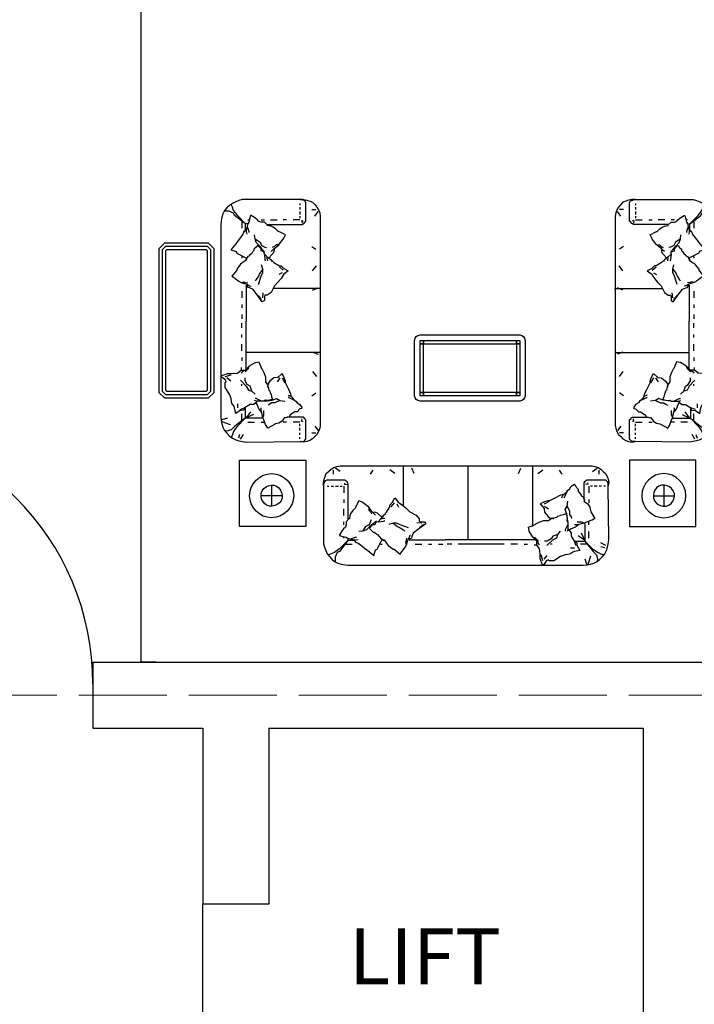
# Model space of a CAD drawing. Units: inches. Extents: x -113 to 5399, y -1393 to 3302.
# Tile 37 of 40: x 3412 to 3504, y 2903 to 3038. Entities that reach past the tile are written whole.
import ezdxf

# ---------------------------------------------------------------- set-up
doc = ezdxf.new("R2010")
doc.units = ezdxf.units.IN
doc.header["$MEASUREMENT"] = 0
doc.linetypes.add('ACAD_ISO02W100', pattern=[15, 12, -3])
doc.layers.add('24', color=7, linetype='Continuous')
for name, color, linetype, lineweight in [('A-ANNO-DIMS', 254, 'Continuous', 18), ('A-AREA-IDEN', 4, 'Continuous', 18), ('doors', 2, 'Continuous', 25), ('furniture', 131, 'Continuous', 18), ('GRIDS', 7, 'ACAD_ISO02W100', 13), ('walls', 1, 'Continuous', 25)]:
    doc.layers.add(name, color=color, linetype=linetype, lineweight=lineweight)
doc.styles.get("Standard").update_dxf_attribs({"font": 'arial.ttf'})
doc.dimstyles.get("Standard").update_dxf_attribs({"dimtxt": 6, "dimasz": 0.18, "dimexe": 0.18, "dimexo": 0.0625, "dimgap": 0.09, "dimtad": 0, "dimtih": 1, "dimtoh": 1, "dimdec": 1, "dimzin": 0, "dimdsep": 46, "dimlunit": 4, "dimtxsty": 'Standard', "dimblk": 'ARCHTICK', "dimcen": 0.09, "dimadec": 0, "dimazin": 0, "dimtfac": 1, "dimtdec": 1, "dimtofl": 0, "dimtmove": 0, "dimatfit": 3, "dimfxl": 1, "dimtolj": 1, "dimtzin": 0, "dimarcsym": 0})

# ---------------------------------------------------------------- blocks, each defined once
blk = doc.blocks.new('*U3')
for p, q in [((0, 0), (0, -6)), ((36, 0), (36, -6))]:
    blk.add_line(p, q)
blk.add_lwpolyline([(0, 0), (0, 36), (1.75, 36), (1.75, 0)], close=True)
blk.add_arc((0, 0), 36, 0, 90)
blk = doc.blocks.new('DL13712')
at = {"layer": '24'}
for p, q in [((33, 28.5), (-34, 28.5)), ((33.5, -29.5), (-10, -29.5))]:
    blk.add_line(p, q, dxfattribs=at)
blk = doc.blocks.new('DL13976')
at = {"layer": '24'}
for p, q in [((-10.5, 16.5), (-7, 18.5)), ((-7, 18.5), (-3.5, 19.5)), ((-3.5, 19.5), (0.5, 20)), ((0.5, 20), (4.5, 19.5)), ((4.5, 19.5), (8, 18.5)), ((8, 18.5), (11.5, 16.5)), ((-18, 7.5), (-16, 11)), ((-16, 11), (-13.5, 14)), ((-13.5, 14), (-10.5, 16.5)), ((-4.5, 8), (-2.5, 9)), ((-2.5, 9), (0, 9.5)), ((0, 9.5), (2.5, 9.5)), ((0.5, -9.5), (0.5, 9.5)), ((2.5, 9.5), (5, 8.5)), ((11.5, 16.5), (14.5, 14)), ((14.5, 14), (17, 11)), ((17, 11), (19, 7.5)), ((-19.5, 0), (-19, 4)), ((-19, -4), (-19.5, 0)), ((-19, 4), (-18, 7.5)), ((-9, 2), (-8, 4.5)), ((-9, -0.5), (-9, 2)), ((-9, 0), (10, 0)), ((-8, 4.5), (-6.5, 6.5)), ((-6.5, 6.5), (-4.5, 8)), ((-5.5, 0), (6.5, 0)), ((0.5, -6), (0.5, 6)), ((5, 8.5), (7, 7)), ((7, 7), (8.5, 5)), ((8.5, 5), (9.5, 3)), ((9.5, 3), (10, 0.5)), ((10, 0.5), (10, -2)), ((19, 7.5), (20, 4)), ((20, 4), (20.5, 0)), ((20.5, 0), (20, -4)), ((-18, -7.5), (-19, -4)), ((-16, -11), (-18, -7.5)), ((-8.5, -3), (-9, -0.5)), ((-7.5, -5), (-8.5, -3)), ((-6, -7), (-7.5, -5)), ((-4, -8.5), (-6, -7)), ((-1.5, -9.5), (-4, -8.5)), ((5.5, -8), (3.5, -9)), ((7.5, -6.5), (5.5, -8)), ((9, -4.5), (7.5, -6.5)), ((10, -2), (9, -4.5)), ((19, -7.5), (17, -11)), ((20, -4), (19, -7.5)), ((-13.5, -14), (-16, -11)), ((-10.5, -16.5), (-13.5, -14)), ((-7, -18.5), (-10.5, -16.5)), ((1, -9.5), (-1.5, -9.5)), ((3.5, -9), (1, -9.5)), ((11.5, -16.5), (8, -18.5)), ((14.5, -14), (11.5, -16.5)), ((17, -11), (14.5, -14)), ((-3.5, -19.5), (-7, -18.5)), ((0.5, -20), (-3.5, -19.5)), ((4.5, -19.5), (0.5, -20)), ((8, -18.5), (4.5, -19.5))]:
    blk.add_line(p, q, dxfattribs=at)
blk = doc.blocks.new('DL13329')
at = {"layer": '24'}
for p, q in [((0, 0), (0, -60)), ((60, 0), (0, 0)), ((60, -60), (60, 0)), ((0, -60), (60, -60))]:
    blk.add_line(p, q, dxfattribs=at)
blk = doc.blocks.new('DL13303')
at = {"layer": '24'}
for p, q in [((-70, 20), (-65, 25)), ((-70, -20), (-70, 20)), ((-67, 19), (-64, 22)), ((-67, -19), (-67, 19)), ((-65, 25), (65, 25)), ((-64, 22), (64, 22)), ((-64, 18), (-63, 19)), ((-64, -18), (-64, 18)), ((-63, 19), (63, 19)), ((63, 19), (64, 18)), ((64, 22), (67, 19)), ((64, 18), (64, -18)), ((65, 25), (70, 20)), ((67, 19), (67, -19)), ((70, 20), (70, -20)), ((-65, -25), (-70, -20)), ((-64, -22), (-67, -19)), ((65, -25), (-65, -25)), ((-63, -19), (-64, -18)), ((64, -22), (-64, -22)), ((63, -19), (-63, -19)), ((64, -18), (63, -19)), ((67, -19), (64, -22)), ((70, -20), (65, -25))]:
    blk.add_line(p, q, dxfattribs=at)
blk = doc.blocks.new('DL12701')
at = {"layer": '24'}
for p, q in [((-93.5, 44.5), (-90, 45)), ((-90, 45), (-87, 45.5)), ((-87, 45.5), (0, 45.5)), ((0, 45.5), (87, 45.5)), ((50, 45), (48, 39.5)), ((51.5, 44.5), (50, 45)), ((87, 45.5), (90.5, 45)), ((90.5, 45), (93.5, 44.5)), ((-106, 35), (-104, 37.5)), ((-102.5, 35), (-105, 36)), ((-104, 37.5), (-102, 40)), ((-102, 40), (-99.5, 42)), ((-99.5, 42), (-96.5, 43.5)), ((-99, 40), (-99, 42)), ((-99, 38), (-99, 40)), ((-98, 36), (-99, 38)), ((-97, 34), (-98, 36)), ((-96.5, 43.5), (-93.5, 44.5)), ((-67.5, 33.5), (-64, 36.5)), ((-64, 36.5), (-62.5, 31.5)), ((48, 39.5), (48, 35.5)), ((50.5, 41.5), (49, 36)), ((53.5, 41.5), (51.5, 44.5)), ((51.5, 40), (54.5, 36.5)), ((55.5, 40.5), (53.5, 41.5)), ((56, 41.5), (55.5, 40.5)), ((60.5, 41.5), (56, 41.5)), ((66.5, 37.5), (60.5, 41.5)), ((70.5, 36), (66.5, 37.5)), ((75, 35.5), (70.5, 36)), ((88.5, 39.5), (90, 44.5)), ((91.5, 44.5), (94, 37)), ((93.5, 44.5), (96.5, 43.5)), ((96.5, 43.5), (99.5, 42)), ((97.5, 34.5), (99, 36)), ((99, 36), (99.5, 38)), ((99.5, 42), (102, 40)), ((100, 40), (99.5, 42)), ((99.5, 38), (100, 40)), ((102, 40), (104.5, 37.5)), ((103, 35), (106, 36)), ((104.5, 37.5), (106.5, 35)), ((-109.5, 26), (-108.5, 29)), ((-108.5, 29), (-107.5, 32)), ((-107.5, 32), (-106, 35)), ((-99.5, 34), (-102.5, 35)), ((-97, 32), (-99.5, 34)), ((-95, 33), (-97, 34)), ((-95, 30.5), (-97, 32)), ((-87.5, 23), (-95, 33)), ((-87.5, 23), (-95, 30.5)), ((-78, 25.5), (-76, 27)), ((-76, 27), (-71.5, 30.5)), ((-71.5, 30.5), (-69.5, 32)), ((-69.5, 32), (-67.5, 33.5)), ((-62.5, 31.5), (-61, 31)), ((-61, 31), (-59.5, 28)), ((-59.5, 28), (-57.5, 24.5)), ((-52, 26.5), (-51, 27.5)), ((-51, 27.5), (-49, 29)), ((-49, 29), (-46.5, 31)), ((-46.5, 31), (-45.5, 31)), ((-45.5, 31), (-40, 35.5)), ((-40, 35.5), (-38.5, 33)), ((-38.5, 33), (-38, 32.5)), ((-38, 32.5), (-35.5, 29)), ((-35.5, 29), (-34.5, 27)), ((-34.5, 27), (-35, 24.5)), ((-34.5, 27), (-33.5, 24)), ((42.5, 27), (45, 27)), ((45.5, 28), (45, 27)), ((45, 27), (45, 23.5)), ((47.5, 30.5), (45.5, 28)), ((46.5, 26), (47.5, 27)), ((48, 35.5), (47.5, 30.5)), ((54, 27.5), (59.5, 22.5)), ((77.5, 33.5), (75, 35.5)), ((79, 30), (75.5, 30)), ((79, 33), (77.5, 33.5)), ((84, 32), (79, 33)), ((80.5, 28), (79, 24)), ((81, 24.5), (81.5, 28)), ((81.5, 28), (84, 32)), ((88.5, 23.5), (96, 33)), ((88.5, 23.5), (95.5, 30.5)), ((95.5, 30.5), (98, 32.5)), ((96, 33), (97.5, 34.5)), ((98, 32.5), (100.5, 34)), ((100.5, 34), (103, 35)), ((103, 28.5), (106.5, 29.5)), ((107.5, 27.5), (103, 25)), ((106.5, 35), (108, 32)), ((108, 32), (109, 29)), ((109, 29), (109.5, 26)), ((-109.5, 22.5), (-109.5, 26)), ((-109.5, -26.5), (-109.5, 22.5)), ((-95, 18.5), (-92, 19.5)), ((-95, 18), (-95, 18.5)), ((-94, 16.5), (-95, 18)), ((-92, 19.5), (-89, 20)), ((-91, 21), (-91, 19.5)), ((-89.5, 26.5), (-83.5, 26.5)), ((-89, 20), (-87.5, 21)), ((-87.5, 21), (-87.5, 23)), ((-81.5, 23), (-87.5, 23)), ((-87.5, 21), (-85, 21.5)), ((-85, 21.5), (-82, 22.5)), ((-85, 21.5), (-80.5, 20)), ((-82, 22.5), (-80.5, 24.5)), ((-82, 22.5), (-80.5, 22.5)), ((-80.5, 24.5), (-78, 25.5)), ((-80.5, 24.5), (-80.5, 23.5)), ((-80.5, 22.5), (-78, 22)), ((-80.5, 20), (-79.5, 20)), ((-77, 25.5), (-77, 25.5)), ((-60.5, 17.5), (-59, 19.5)), ((-59, 19.5), (-58.5, 19.5)), ((-58.5, 19.5), (-58, 21)), ((-58, 26.5), (-56.5, 26.5)), ((-58, 21), (-54.5, 23)), ((-57.5, 24.5), (-56.5, 22)), ((-56.5, 22.5), (-54.5, 22.5)), ((-54.5, 22.5), (-52.5, 25.5)), ((-54.5, 23), (-54.5, 22.5)), ((-54, 22.5), (-54, 22.5)), ((-52.5, 25.5), (-52, 26.5)), ((-35, 24.5), (-34.5, 23)), ((-34.5, 23), (-34, 21)), ((-33.5, 24), (-33, 22)), ((-30, 21), (-33, 22)), ((-33, 22), (-31.5, 19.5)), ((-32, 22.5), (0.5, 22.5)), ((-31.5, 19.5), (-31, 18)), ((-29.5, 19.5), (-30, 21)), ((-28.5, 16.5), (-29.5, 19.5)), ((-26.5, 26.5), (-20.5, 26.5)), ((-14.5, 26.5), (-11.5, 26.5)), ((-5.5, 26.5), (-1.5, 26.5)), ((44, 22.5), (0.5, 22.5)), ((6.5, 26.5), (2.5, 26.5)), ((15.5, 26.5), (12.5, 26.5)), ((27.5, 26.5), (21.5, 26.5)), ((33.5, 26.5), (36.5, 26.5)), ((40.5, 18.5), (38, 14.5)), ((41.5, 20), (40.5, 18.5)), ((43.5, 22), (41.5, 20)), ((43.5, 20.5), (41.5, 20)), ((45, 23.5), (43.5, 22)), ((45, 22), (43.5, 20.5)), ((45, 23.5), (46.5, 26)), ((46.5, 23.5), (45, 22)), ((54.5, 23.5), (52, 23.5)), ((58, 21.5), (54.5, 23.5)), ((59, 26.5), (57.5, 26.5)), ((59.5, 19), (58, 21.5)), ((59.5, 22.5), (63, 20.5)), ((64, 17.5), (59.5, 19)), ((63, 20.5), (64, 17.5)), ((76, 19), (79, 24)), ((76, 16), (76, 19)), ((79, 24), (81, 24.5)), ((79, 23.5), (88.5, 23.5)), ((82.5, 18.5), (88, 22.5)), ((90.5, 26.5), (84.5, 26.5)), ((85, 16), (88, 22.5)), ((88.5, 8), (88.5, 23.5)), ((92, 21), (92, 15)), ((109.5, 26), (110, 22.5)), ((110, 22.5), (109.5, -26.5)), ((-92.5, 14), (-94, 16.5)), ((-92, 13.5), (-92.5, 14)), ((-91.5, 12.5), (-92, 13.5)), ((-89.5, 11), (-91.5, 12.5)), ((-91, 9), (-91, 6)), ((-89, 9), (-89.5, 11)), ((-89, 8.5), (-89, 9)), ((-74, 14.5), (-77.5, 15)), ((-70.5, 13.5), (-74, 14.5)), ((-74, 14.5), (-71, 10)), ((-71, 10), (-68, 8.5)), ((-67.5, 10.5), (-70.5, 13.5)), ((-68, 12), (-67.5, 12.5)), ((-65, 9), (-68, 12)), ((-67.5, 12.5), (-66.5, 13.5)), ((-61.5, 5.5), (-67.5, 10.5)), ((-66.5, 13.5), (-64.5, 15.5)), ((-63, 9), (-65, 9)), ((-64.5, 15.5), (-63.5, 15.5)), ((-63.5, 15.5), (-62.5, 16.5)), ((-62, 6.5), (-63, 9)), ((-62.5, 16.5), (-60.5, 17.5)), ((-46.5, 7.5), (-42.5, 10.5)), ((-40, 9), (-43.5, 7.5)), ((-42.5, 10.5), (-40, 11.5)), ((-40, 11.5), (-37, 13.5)), ((-32.5, 11.5), (-40, 9)), ((-37, 13.5), (-36, 14.5)), ((-24.5, 13.5), (-28.5, 16.5)), ((-21, 11), (-24.5, 13.5)), ((-19, 8.5), (-22.5, 11.5)), ((-17, 8), (-21, 11)), ((38, 14), (37.5, 11)), ((37.5, 11), (43.5, 8.5)), ((38, 14.5), (38, 14)), ((64, 17.5), (66.5, 14.5)), ((70.5, 13.5), (70.5, 14.5)), ((73, 8.5), (70.5, 13.5)), ((73, 13), (72.5, 15)), ((73, 12.5), (75, 14.5)), ((73, 12.5), (73, 13)), ((73, 8.5), (73, 12.5)), ((76, 12.5), (74, 14)), ((75, 14.5), (76, 16)), ((75.5, 16), (76, 16.5)), ((80, 11), (76, 12.5)), ((80.5, 9), (79, 9)), ((80.5, 10.5), (80, 11)), ((83, 8.5), (80.5, 10.5)), ((83, 8.5), (80.5, 9)), ((92, 9), (92, 6)), ((-91, 0.5), (-91, -5.5)), ((-89, 6), (-89, 8.5)), ((-86.5, 3.5), (-89, 6)), ((-87, 3.5), (-87, -26.5)), ((-86, 3.5), (-86.5, 3.5)), ((-85.5, 0.5), (-86, 3.5)), ((-85.5, 0), (-85.5, 0.5)), ((-84.5, -2), (-85.5, 0)), ((-68, 8.5), (-66.5, 5.5)), ((-66.5, 5.5), (-66, 4)), ((-62.5, 0), (-63.5, -1)), ((-60, 6), (-62, 6.5)), ((-61, -2), (-58.5, 0.5)), ((-57.5, 3.5), (-60, 6)), ((-60, 6), (-55, 5.5)), ((-58.5, 0.5), (-55.5, 2)), ((-56.5, 3.5), (-57.5, 3.5)), ((-57.5, 3.5), (-56, 1.5)), ((-54, 3), (-56.5, 3.5)), ((-56, 1.5), (-55, 0)), ((-55, 5.5), (-54, 5)), ((-55, 0), (-52.5, -2.5)), ((-46.5, 7.5), (-50.5, 8.5)), ((-43.5, 7.5), (-46.5, 7.5)), ((-31.5, -3), (-25.5, 0)), ((-25.5, 0), (-23, 3.5)), ((-20.5, 7.5), (-25, 7)), ((-23, 5.5), (-21.5, 6)), ((-23, 3.5), (-23, 5.5)), ((-21.5, 6), (-18, 6)), ((-18, 6), (-17, 8)), ((43.5, 8.5), (44, 8)), ((44, 8), (47, 6.5)), ((47, 6.5), (49.5, 5.5)), ((49.5, 5.5), (51, 5)), ((51, 5), (52.5, 5)), ((52, -2.5), (55, 1)), ((52.5, 5), (55.5, 5)), ((55, 1), (57.5, 3)), ((55.5, 5), (55.5, 5)), ((55.5, 5), (59, 2.5)), ((59, 2.5), (60, 3.5)), ((60, 3.5), (60, 2.5)), ((60, 2.5), (63, 2)), ((63, 2), (64, 1)), ((64, 1), (66, 0.5)), ((66, 0.5), (66.5, 0)), ((66.5, 0), (69, -0.5)), ((71.5, -1), (72.5, 2.5)), ((72, 5), (73, 6.5)), ((73, 5.5), (72, -1)), ((72.5, 2.5), (72, 5)), ((73, 6.5), (73, 8.5)), ((74.5, -0.5), (76, 1.5)), ((76, 1.5), (76.5, 3)), ((84, 6.5), (81.5, 6.5)), ((85, 8), (83, 8.5)), ((85.5, 6.5), (84, 6.5)), ((88, 7.5), (85, 8)), ((88, 7.5), (85.5, 6.5)), ((90, 6.5), (88, 7.5)), ((94, 5), (90, 6.5)), ((95, 4.5), (94, 5)), ((94, -3), (97.5, 3)), ((97.5, 3), (95, 4.5)), ((-83, -4), (-84.5, -2)), ((-80.5, -6.5), (-83, -4)), ((-80.5, -7), (-80.5, -6.5)), ((-77.5, -13), (-80.5, -7)), ((-70.5, -8.5), (-73.5, -11)), ((-68.5, -7), (-70.5, -8.5)), ((-68.5, -4.5), (-67, -3)), ((-66.5, -4.5), (-68.5, -7)), ((-68.5, -7), (-68.5, -4.5)), ((-67, -3), (-66, -1)), ((-65.5, -3), (-66.5, -4.5)), ((-63.5, -1), (-65.5, -3)), ((-65.5, -3), (-62.5, -2.5)), ((-62.5, -2.5), (-61, -2)), ((-54, -0.5), (-53.5, -0.5)), ((-52.5, -2.5), (-49.5, -7.5)), ((-49.5, -7.5), (-49.5, -9)), ((-45.5, -11), (-48.5, -7.5)), ((-43, -10), (-41.5, -7)), ((-38, -9), (-35, -6.5)), ((-35, -6.5), (-31.5, -3)), ((48, -10), (51.5, -6)), ((51.5, -5.5), (52, -2.5)), ((51.5, -6), (51.5, -5.5)), ((52, -8), (55.5, -5.5)), ((69, -0.5), (70.5, -1)), ((70.5, -1), (71.5, -1)), ((72, -1), (70.5, -5)), ((70.5, -5), (72.5, -8)), ((72.5, -8), (74.5, -3.5)), ((72.5, -8), (73, -12.5)), ((74.5, -3.5), (74.5, -0.5)), ((91, -10), (92, -8.5)), ((92, -8.5), (93, -7)), ((93, -7), (93.5, -4)), ((93.5, -4), (94, -3)), ((-91, -14), (-91, -11)), ((-74.5, -11.5), (-77.5, -13)), ((-73.5, -11), (-74.5, -11.5)), ((-49.5, -9), (-47, -11.5)), ((-47, -11.5), (-45, -15.5)), ((-45, -15.5), (-42, -11.5)), ((-42, -11.5), (-41, -11)), ((-41, -11), (-38, -9)), ((52, -12), (48, -10)), ((52, -10), (56.5, -12.5)), ((55, -13), (52, -12)), ((56.5, -13), (55, -13)), ((62.5, -16), (56.5, -13)), ((64.5, -17), (62.5, -16)), ((64, -16.5), (64, -16.5)), ((66.5, -18), (64.5, -17)), ((67.5, -15.5), (68.5, -18)), ((70, -16.5), (69.5, -15.5)), ((72, -21), (70, -16.5)), ((85, -17.5), (87, -16.5)), ((85, -18), (85, -17.5)), ((87, -16.5), (88, -13)), ((87.5, -12.5), (89.5, -11)), ((88, -13), (87.5, -12.5)), ((87.5, -26.5), (87.5, -14.5)), ((89.5, -11), (91, -10)), ((92, -14), (92, -11)), ((-109.5, -28), (-109.5, -26.5)), ((-109.5, -26.5), (-109.5, -29.5)), ((-106, -26), (-104.5, -26)), ((-102.5, -26), (-100.5, -26)), ((-98.5, -26), (-96, -26)), ((-94.5, -26), (-92.5, -26)), ((-91, -26), (-91, -20)), ((-87, -26.5), (-87, -28)), ((69, -18.5), (66.5, -18)), ((68.5, -18), (69, -18.5)), ((69, -18.5), (72, -21)), ((72, -21), (73, -22.5)), ((73, -22.5), (74.5, -23.5)), ((74.5, -23.5), (76, -26)), ((76, -26), (79, -28)), ((79.5, -27.5), (80, -26)), ((80, -26), (82.5, -23.5)), ((82.5, -21.5), (83.5, -20)), ((82.5, -22.5), (82.5, -21.5)), ((82.5, -23.5), (82.5, -22.5)), ((83.5, -20), (85, -18)), ((87.5, -28), (87.5, -26.5)), ((92, -26), (92, -20)), ((95.5, -26), (93.5, -26)), ((99.5, -26), (97, -26)), ((103.5, -26), (101.5, -26)), ((107, -26), (105.5, -26)), ((110, -29.5), (109.5, -26.5)), ((109.5, -26.5), (109.5, -28)), ((-109, -29), (-109.5, -28)), ((-109.5, -29.5), (-109, -32.5)), ((-108.5, -30), (-109, -29)), ((-109, -32.5), (-108, -35)), ((-108, -31), (-108.5, -30)), ((-106.5, -31.5), (-108, -31)), ((-108, -35), (-107, -37.5)), ((-105.5, -31.5), (-106.5, -31.5)), ((-104.5, -31.5), (-105.5, -31.5)), ((-92, -31.5), (-104.5, -31.5)), ((-91, -31.5), (-92, -31.5)), ((-90, -31.5), (-91, -31.5)), ((-90.5, -27.5), (-88, -28)), ((-90.5, -28), (-90, -29)), ((-89, -30.5), (-90, -31.5)), ((-88, -30), (-89, -30.5)), ((-87.5, -29), (-88, -30)), ((-87, -28), (-87.5, -29)), ((79, -28), (79.5, -27.5)), ((87.5, -29), (87.5, -28)), ((88, -30), (87.5, -29)), ((89, -30.5), (88, -30)), ((91.5, -27.5), (89, -28)), ((90, -31.5), (89, -30.5)), ((91, -31.5), (90, -31.5)), ((91.5, -28), (91, -29)), ((92.5, -31.5), (91, -31.5)), ((104.5, -31.5), (92.5, -31.5)), ((106, -31.5), (104.5, -31.5)), ((107, -31.5), (106, -31.5)), ((108, -31), (107, -31.5)), ((107, -37.5), (108.5, -35)), ((109, -30), (108, -31)), ((108.5, -35), (109.5, -32.5)), ((109.5, -29), (109, -30)), ((109.5, -28), (109.5, -29)), ((109.5, -32.5), (110, -29.5)), ((-107, -37.5), (-105, -39.5)), ((-105, -39.5), (-102.5, -41.5)), ((-102.5, -41.5), (-100, -43)), ((-100.5, -37), (-100.5, -40.5)), ((-100, -43), (-97.5, -44)), ((-94.5, -39.5), (-98.5, -42.5)), ((-97.5, -44), (-94.5, -44.5)), ((-94.5, -44.5), (0, -44.5)), ((-67, -37), (-64.5, -40.5)), ((-45, -37.5), (-49.5, -41)), ((-27.5, -37.5), (-29.5, -42.5)), ((0, -44.5), (95, -44.5)), ((28.5, -37.5), (30.5, -42.5)), ((46, -37.5), (50.5, -41)), ((68, -37), (65.5, -40.5)), ((95, -44.5), (97.5, -44)), ((95.5, -39.5), (99.5, -42.5)), ((97.5, -44), (100.5, -43)), ((100.5, -43), (103, -41.5)), ((101.5, -37), (101.5, -40.5)), ((103, -41.5), (105, -39.5)), ((105, -39.5), (107, -37.5))]:
    blk.add_line(p, q, dxfattribs=at)
blk = doc.blocks.new('DL13707')
at = {"layer": '24'}
for p, q in [((0, -33.5), (0, 33.5)), ((-58.5, -33.5), (-58.5, 21.5)), ((58.5, -33.5), (58.5, 2))]:
    blk.add_line(p, q, dxfattribs=at)
blk = doc.blocks.new('DL13651')
at = {"layer": '24'}
for p, q in [((-50.5, 25), (-50, 27)), ((-50, 27), (-49, 28.5)), ((-49, 28.5), (-47.5, 29.5)), ((-47.5, 29.5), (-45.5, 30)), ((-45.5, 30), (44.5, 30)), ((44.5, 30), (46.5, 29.5)), ((46.5, 29.5), (48, 28.5)), ((48, 28.5), (49, 27)), ((49, 27), (49.5, 25)), ((-50.5, -25), (-50.5, 25)), ((-45.5, 24.5), (-45.5, 25)), ((-45.5, 25), (-45, 25)), ((-45.5, -24.5), (-45.5, 24.5)), ((-45, 25), (44, 25)), ((-45, 22), (44, 22)), ((-42.5, 22), (-45, 22)), ((-42.5, -24.5), (-42.5, 24.5)), ((-42.5, 24.5), (-42.5, 22)), ((41.5, 22), (41.5, 24.5)), ((41.5, 24.5), (41.5, -24.5)), ((44, 22), (41.5, 22)), ((44, 25), (44.5, 25)), ((44.5, 25), (44.5, 24.5)), ((44.5, 24.5), (44.5, -24.5)), ((49.5, 25), (49.5, -25)), ((-50, -27), (-50.5, -25)), ((-45.5, -25), (-45.5, -24.5)), ((-45, -25), (-45.5, -25)), ((44, -22), (-45, -22)), ((-45, -22), (-42.5, -22)), ((44, -25), (-45, -25)), ((-42.5, -22), (-42.5, -24.5)), ((41.5, -24.5), (41.5, -22)), ((41.5, -22), (44, -22)), ((44.5, -25), (44, -25)), ((44.5, -24.5), (44.5, -25)), ((49.5, -25), (49, -27)), ((-49, -28.5), (-50, -27)), ((-47.5, -29.5), (-49, -28.5)), ((-45.5, -30), (-47.5, -29.5)), ((44.5, -30), (-45.5, -30)), ((46.5, -29.5), (44.5, -30)), ((48, -28.5), (46.5, -29.5)), ((49, -27), (48, -28.5))]:
    blk.add_line(p, q, dxfattribs=at)
blk = doc.blocks.new('DL12263')
at = {"layer": '24'}
for p, q in [((-112.5, 44.5), (-109, 45)), ((-109, 45), (-106, 45.5)), ((-106, 45.5), (-19, 45.5)), ((-19, 45.5), (106.5, 45.5)), ((69.5, 45), (67.5, 39.5)), ((71, 44.5), (69.5, 45)), ((106.5, 45.5), (110, 45)), ((110, 45), (113, 44.5)), ((-125, 35), (-123, 37.5)), ((-121.5, 35), (-124, 36)), ((-123, 37.5), (-121, 40)), ((-121, 40), (-118.5, 42)), ((-118.5, 42), (-115.5, 43.5)), ((-118, 40), (-118, 42)), ((-118, 38), (-118, 40)), ((-117, 36), (-118, 38)), ((-116, 34), (-117, 36)), ((-115.5, 43.5), (-112.5, 44.5)), ((-86.5, 33.5), (-83, 36.5)), ((-83, 36.5), (-81.5, 31.5)), ((67.5, 39.5), (67.5, 35.5)), ((70, 41.5), (68.5, 36)), ((73, 41.5), (71, 44.5)), ((71, 40), (74, 36.5)), ((75, 40.5), (73, 41.5)), ((75.5, 41.5), (75, 40.5)), ((80, 41.5), (75.5, 41.5)), ((86, 37.5), (80, 41.5)), ((90, 36), (86, 37.5)), ((94.5, 35.5), (90, 36)), ((108, 39.5), (109.5, 44.5)), ((111, 44.5), (113.5, 37)), ((113, 44.5), (116, 43.5)), ((116, 43.5), (119, 42)), ((117, 34.5), (118.5, 36)), ((118.5, 36), (119, 38)), ((119, 42), (121.5, 40)), ((119.5, 40), (119, 42)), ((119, 38), (119.5, 40)), ((121.5, 40), (124, 37.5)), ((122.5, 35), (125.5, 36)), ((124, 37.5), (126, 35)), ((-128.5, 26), (-127.5, 29)), ((-127.5, 29), (-126.5, 32)), ((-126.5, 32), (-125, 35)), ((-118.5, 34), (-121.5, 35)), ((-116, 32), (-118.5, 34)), ((-114, 33), (-116, 34)), ((-114, 30.5), (-116, 32)), ((-106.5, 23), (-114, 33)), ((-106.5, 23), (-114, 30.5)), ((-97, 25.5), (-95, 27)), ((-95, 27), (-90.5, 30.5)), ((-90.5, 30.5), (-88.5, 32)), ((-88.5, 32), (-86.5, 33.5)), ((-81.5, 31.5), (-80, 31)), ((-80, 31), (-78.5, 28)), ((-78.5, 28), (-76.5, 24.5)), ((-71, 26.5), (-70, 27.5)), ((-70, 27.5), (-68, 29)), ((-68, 29), (-65.5, 31)), ((-65.5, 31), (-64.5, 31)), ((-64.5, 31), (-59, 35.5)), ((-59, 35.5), (-57.5, 33)), ((-57.5, 33), (-57, 32.5)), ((-57, 32.5), (-54.5, 29)), ((-54.5, 29), (-53.5, 27)), ((-53.5, 27), (-54, 24.5)), ((-53.5, 27), (-52.5, 24)), ((62, 27), (64.5, 27)), ((65, 28), (64.5, 27)), ((64.5, 27), (64.5, 23.5)), ((67, 30.5), (65, 28)), ((66, 26), (67, 27)), ((67.5, 35.5), (67, 30.5)), ((73.5, 27.5), (79, 22.5)), ((97, 33.5), (94.5, 35.5)), ((98.5, 30), (95, 30)), ((98.5, 33), (97, 33.5)), ((103.5, 32), (98.5, 33)), ((100, 28), (98.5, 24)), ((100.5, 24.5), (101, 28)), ((101, 28), (103.5, 32)), ((108, 23.5), (115.5, 33)), ((108, 23.5), (115, 30.5)), ((115, 30.5), (117.5, 32.5)), ((115.5, 33), (117, 34.5)), ((117.5, 32.5), (120, 34)), ((120, 34), (122.5, 35)), ((122.5, 28.5), (126, 29.5)), ((127, 27.5), (122.5, 25)), ((126, 35), (127.5, 32)), ((127.5, 32), (128.5, 29)), ((128.5, 29), (129, 26)), ((-128.5, 22.5), (-128.5, 26)), ((-128.5, -26.5), (-128.5, 22.5)), ((-114, 18.5), (-111, 19.5)), ((-114, 18), (-114, 18.5)), ((-113, 16.5), (-114, 18)), ((-111, 19.5), (-108, 20)), ((-110, 21), (-110, 19.5)), ((-108.5, 26.5), (-102.5, 26.5)), ((-108, 20), (-106.5, 21)), ((-106.5, 21), (-106.5, 23)), ((-100.5, 23), (-106.5, 23)), ((-106.5, 21), (-104, 21.5)), ((-104, 21.5), (-101, 22.5)), ((-104, 21.5), (-99.5, 20)), ((-101, 22.5), (-99.5, 24.5)), ((-101, 22.5), (-99.5, 22.5)), ((-99.5, 24.5), (-97, 25.5)), ((-99.5, 24.5), (-99.5, 23.5)), ((-99.5, 22.5), (-97, 22)), ((-99.5, 20), (-98.5, 20)), ((-96, 25.5), (-96, 25.5)), ((-79.5, 17.5), (-78, 19.5)), ((-78, 19.5), (-77.5, 19.5)), ((-77.5, 19.5), (-77, 21)), ((-77, 26.5), (-75.5, 26.5)), ((-77, 21), (-73.5, 23)), ((-76.5, 24.5), (-75.5, 22)), ((-75.5, 22.5), (-73.5, 22.5)), ((-73.5, 22.5), (-71.5, 25.5)), ((-73.5, 23), (-73.5, 22.5)), ((-73, 22.5), (-73, 22.5)), ((-71.5, 25.5), (-71, 26.5)), ((-54, 24.5), (-53.5, 23)), ((-53.5, 23), (-53, 21)), ((-52.5, 24), (-52, 22)), ((-49, 21), (-52, 22)), ((-52, 22), (-50.5, 19.5)), ((-51, 22.5), (-18.5, 22.5)), ((-50.5, 19.5), (-50, 18)), ((-48.5, 19.5), (-49, 21)), ((-47.5, 16.5), (-48.5, 19.5)), ((-45.5, 26.5), (-39.5, 26.5)), ((-33.5, 26.5), (-30.5, 26.5)), ((-24.5, 26.5), (-20.5, 26.5)), ((63.5, 22.5), (-18.5, 22.5)), ((-12.5, 26.5), (-16.5, 26.5)), ((35, 26.5), (-6.5, 26.5)), ((47, 26.5), (41, 26.5)), ((53, 26.5), (56, 26.5)), ((60, 18.5), (57.5, 14.5)), ((61, 20), (60, 18.5)), ((63, 22), (61, 20)), ((63, 20.5), (61, 20)), ((64.5, 23.5), (63, 22)), ((64.5, 22), (63, 20.5)), ((64.5, 23.5), (66, 26)), ((66, 23.5), (64.5, 22)), ((74, 23.5), (71.5, 23.5)), ((77.5, 21.5), (74, 23.5)), ((78.5, 26.5), (77, 26.5)), ((79, 19), (77.5, 21.5)), ((79, 22.5), (82.5, 20.5)), ((83.5, 17.5), (79, 19)), ((82.5, 20.5), (83.5, 17.5)), ((95.5, 19), (98.5, 24)), ((95.5, 16), (95.5, 19)), ((98.5, 24), (100.5, 24.5)), ((98.5, 23.5), (108, 23.5)), ((102, 18.5), (107.5, 22.5)), ((110, 26.5), (104, 26.5)), ((104.5, 16), (107.5, 22.5)), ((108, 8), (108, 23.5)), ((111.5, 21), (111.5, 15)), ((129, 26), (129.5, 22.5)), ((129.5, 22.5), (129, -26.5)), ((-111.5, 14), (-113, 16.5)), ((-111, 13.5), (-111.5, 14)), ((-110.5, 12.5), (-111, 13.5)), ((-108.5, 11), (-110.5, 12.5)), ((-110, 9), (-110, 6)), ((-108, 9), (-108.5, 11)), ((-108, 8.5), (-108, 9)), ((-93, 14.5), (-96.5, 15)), ((-89.5, 13.5), (-93, 14.5)), ((-93, 14.5), (-90, 10)), ((-90, 10), (-87, 8.5)), ((-86.5, 10.5), (-89.5, 13.5)), ((-87, 12), (-86.5, 12.5)), ((-84, 9), (-87, 12)), ((-86.5, 12.5), (-85.5, 13.5)), ((-80.5, 5.5), (-86.5, 10.5)), ((-85.5, 13.5), (-83.5, 15.5)), ((-82, 9), (-84, 9)), ((-83.5, 15.5), (-82.5, 15.5)), ((-82.5, 15.5), (-81.5, 16.5)), ((-81, 6.5), (-82, 9)), ((-81.5, 16.5), (-79.5, 17.5)), ((-65.5, 7.5), (-61.5, 10.5)), ((-59, 9), (-62.5, 7.5)), ((-61.5, 10.5), (-59, 11.5)), ((-59, 11.5), (-56, 13.5)), ((-51.5, 11.5), (-59, 9)), ((-56, 13.5), (-55, 14.5)), ((-43.5, 13.5), (-47.5, 16.5)), ((-40, 11), (-43.5, 13.5)), ((-38, 8.5), (-41.5, 11.5)), ((-36, 8), (-40, 11)), ((57.5, 14), (57, 11)), ((57, 11), (63, 8.5)), ((57.5, 14.5), (57.5, 14)), ((83.5, 17.5), (86, 14.5)), ((90, 13.5), (90, 14.5)), ((92.5, 8.5), (90, 13.5)), ((92.5, 13), (92, 15)), ((92.5, 12.5), (94.5, 14.5)), ((92.5, 12.5), (92.5, 13)), ((92.5, 8.5), (92.5, 12.5)), ((95.5, 12.5), (93.5, 14)), ((94.5, 14.5), (95.5, 16)), ((95, 16), (95.5, 16.5)), ((99.5, 11), (95.5, 12.5)), ((100, 9), (98.5, 9)), ((100, 10.5), (99.5, 11)), ((102.5, 8.5), (100, 10.5)), ((102.5, 8.5), (100, 9)), ((111.5, 9), (111.5, 6)), ((-110, 0.5), (-110, -5.5)), ((-108, 6), (-108, 8.5)), ((-105.5, 3.5), (-108, 6)), ((-106, 3.5), (-106, -26.5)), ((-105, 3.5), (-105.5, 3.5)), ((-104.5, 0.5), (-105, 3.5)), ((-104.5, 0), (-104.5, 0.5)), ((-103.5, -2), (-104.5, 0)), ((-87, 8.5), (-85.5, 5.5)), ((-85.5, 5.5), (-85, 4)), ((-81.5, 0), (-82.5, -1)), ((-79, 6), (-81, 6.5)), ((-80, -2), (-77.5, 0.5)), ((-76.5, 3.5), (-79, 6)), ((-79, 6), (-74, 5.5)), ((-77.5, 0.5), (-74.5, 2)), ((-75.5, 3.5), (-76.5, 3.5)), ((-76.5, 3.5), (-75, 1.5)), ((-73, 3), (-75.5, 3.5)), ((-75, 1.5), (-74, 0)), ((-74, 5.5), (-73, 5)), ((-74, 0), (-71.5, -2.5)), ((-65.5, 7.5), (-69.5, 8.5)), ((-62.5, 7.5), (-65.5, 7.5)), ((-50.5, -3), (-44.5, 0)), ((-44.5, 0), (-42, 3.5)), ((-39.5, 7.5), (-44, 7)), ((-42, 5.5), (-40.5, 6)), ((-42, 3.5), (-42, 5.5)), ((-40.5, 6), (-37, 6)), ((-37, 6), (-36, 8)), ((63, 8.5), (63.5, 8)), ((63.5, 8), (66.5, 6.5)), ((66.5, 6.5), (69, 5.5)), ((69, 5.5), (70.5, 5)), ((70.5, 5), (72, 5)), ((71.5, -2.5), (74.5, 1)), ((72, 5), (75, 5)), ((74.5, 1), (77, 3)), ((75, 5), (75, 5)), ((75, 5), (78.5, 2.5)), ((78.5, 2.5), (79.5, 3.5)), ((79.5, 3.5), (79.5, 2.5)), ((79.5, 2.5), (82.5, 2)), ((82.5, 2), (83.5, 1)), ((83.5, 1), (85.5, 0.5)), ((85.5, 0.5), (86, 0)), ((86, 0), (88.5, -0.5)), ((91, -1), (92, 2.5)), ((91.5, 5), (92.5, 6.5)), ((92.5, 5.5), (91.5, -1)), ((92, 2.5), (91.5, 5)), ((92.5, 6.5), (92.5, 8.5)), ((94, -0.5), (95.5, 1.5)), ((95.5, 1.5), (96, 3)), ((103.5, 6.5), (101, 6.5)), ((104.5, 8), (102.5, 8.5)), ((105, 6.5), (103.5, 6.5)), ((107.5, 7.5), (104.5, 8)), ((107.5, 7.5), (105, 6.5)), ((109.5, 6.5), (107.5, 7.5)), ((113.5, 5), (109.5, 6.5)), ((114.5, 4.5), (113.5, 5)), ((113.5, -3), (117, 3)), ((117, 3), (114.5, 4.5)), ((-102, -4), (-103.5, -2)), ((-99.5, -6.5), (-102, -4)), ((-99.5, -7), (-99.5, -6.5)), ((-96.5, -13), (-99.5, -7)), ((-89.5, -8.5), (-92.5, -11)), ((-87.5, -7), (-89.5, -8.5)), ((-87.5, -4.5), (-86, -3)), ((-85.5, -4.5), (-87.5, -7)), ((-87.5, -7), (-87.5, -4.5)), ((-86, -3), (-85, -1)), ((-84.5, -3), (-85.5, -4.5)), ((-82.5, -1), (-84.5, -3)), ((-84.5, -3), (-81.5, -2.5)), ((-81.5, -2.5), (-80, -2)), ((-73, -0.5), (-72.5, -0.5)), ((-71.5, -2.5), (-68.5, -7.5)), ((-68.5, -7.5), (-68.5, -9)), ((-64.5, -11), (-67.5, -7.5)), ((-62, -10), (-60.5, -7)), ((-57, -9), (-54, -6.5)), ((-54, -6.5), (-50.5, -3)), ((67.5, -10), (71, -6)), ((71, -5.5), (71.5, -2.5)), ((71, -6), (71, -5.5)), ((71.5, -8), (75, -5.5)), ((88.5, -0.5), (90, -1)), ((90, -1), (91, -1)), ((91.5, -1), (90, -5)), ((90, -5), (92, -8)), ((92, -8), (94, -3.5)), ((92, -8), (92.5, -12.5)), ((94, -3.5), (94, -0.5)), ((110.5, -10), (111.5, -8.5)), ((111.5, -8.5), (112.5, -7)), ((112.5, -7), (113, -4)), ((113, -4), (113.5, -3)), ((-110, -14), (-110, -11)), ((-93.5, -11.5), (-96.5, -13)), ((-92.5, -11), (-93.5, -11.5)), ((-68.5, -9), (-66, -11.5)), ((-66, -11.5), (-64, -15.5)), ((-64, -15.5), (-61, -11.5)), ((-61, -11.5), (-60, -11)), ((-60, -11), (-57, -9)), ((71.5, -12), (67.5, -10)), ((71.5, -10), (76, -12.5)), ((74.5, -13), (71.5, -12)), ((76, -13), (74.5, -13)), ((82, -16), (76, -13)), ((84, -17), (82, -16)), ((83.5, -16.5), (83.5, -16.5)), ((86, -18), (84, -17)), ((87, -15.5), (88, -18)), ((89.5, -16.5), (89, -15.5)), ((91.5, -21), (89.5, -16.5)), ((104.5, -17.5), (106.5, -16.5)), ((104.5, -18), (104.5, -17.5)), ((106.5, -16.5), (107.5, -13)), ((107, -12.5), (109, -11)), ((107.5, -13), (107, -12.5)), ((107, -26.5), (107, -14.5)), ((109, -11), (110.5, -10)), ((111.5, -14), (111.5, -11)), ((-128.5, -28), (-128.5, -26.5)), ((-128.5, -26.5), (-128.5, -29.5)), ((-125, -26), (-123.5, -26)), ((-121.5, -26), (-119.5, -26)), ((-117.5, -26), (-115, -26)), ((-113.5, -26), (-111.5, -26)), ((-110, -26), (-110, -20)), ((-106, -26.5), (-106, -28)), ((88.5, -18.5), (86, -18)), ((88, -18), (88.5, -18.5)), ((88.5, -18.5), (91.5, -21)), ((91.5, -21), (92.5, -22.5)), ((92.5, -22.5), (94, -23.5)), ((94, -23.5), (95.5, -26)), ((95.5, -26), (98.5, -28)), ((99, -27.5), (99.5, -26)), ((99.5, -26), (102, -23.5)), ((102, -21.5), (103, -20)), ((102, -22.5), (102, -21.5)), ((102, -23.5), (102, -22.5)), ((103, -20), (104.5, -18)), ((107, -28), (107, -26.5)), ((111.5, -26), (111.5, -20)), ((115, -26), (113, -26)), ((119, -26), (116.5, -26)), ((123, -26), (121, -26)), ((126.5, -26), (125, -26)), ((129.5, -29.5), (129, -26.5)), ((129, -26.5), (129, -28)), ((-128, -29), (-128.5, -28)), ((-128.5, -29.5), (-128, -32.5)), ((-127.5, -30), (-128, -29)), ((-128, -32.5), (-127, -35)), ((-127, -31), (-127.5, -30)), ((-125.5, -31.5), (-127, -31)), ((-127, -35), (-126, -37.5)), ((-124.5, -31.5), (-125.5, -31.5)), ((-123.5, -31.5), (-124.5, -31.5)), ((-111, -31.5), (-123.5, -31.5)), ((-110, -31.5), (-111, -31.5)), ((-109, -31.5), (-110, -31.5)), ((-109.5, -27.5), (-107, -28)), ((-109.5, -28), (-109, -29)), ((-108, -30.5), (-109, -31.5)), ((-107, -30), (-108, -30.5)), ((-106.5, -29), (-107, -30)), ((-106, -28), (-106.5, -29)), ((98.5, -28), (99, -27.5)), ((107, -29), (107, -28)), ((107.5, -30), (107, -29)), ((108.5, -30.5), (107.5, -30)), ((111, -27.5), (108.5, -28)), ((109.5, -31.5), (108.5, -30.5)), ((110.5, -31.5), (109.5, -31.5)), ((111, -28), (110.5, -29)), ((112, -31.5), (110.5, -31.5)), ((124, -31.5), (112, -31.5)), ((125.5, -31.5), (124, -31.5)), ((126.5, -31.5), (125.5, -31.5)), ((127.5, -31), (126.5, -31.5)), ((126.5, -37.5), (128, -35)), ((128.5, -30), (127.5, -31)), ((128, -35), (129, -32.5)), ((129, -29), (128.5, -30)), ((129, -28), (129, -29)), ((129, -32.5), (129.5, -29.5)), ((-126, -37.5), (-124, -39.5)), ((-124, -39.5), (-121.5, -41.5)), ((-121.5, -41.5), (-119, -43)), ((-119.5, -37), (-119.5, -40.5)), ((-119, -43), (-116.5, -44)), ((-113.5, -39.5), (-117.5, -42.5)), ((-116.5, -44), (-113.5, -44.5)), ((-113.5, -44.5), (-19, -44.5)), ((-86, -37), (-83.5, -40.5)), ((-64, -37.5), (-68.5, -41)), ((-46.5, -37.5), (-48.5, -42.5)), ((-19, -44.5), (114.5, -44.5)), ((48, -37.5), (50, -42.5)), ((65.5, -37.5), (70, -41)), ((87.5, -37), (85, -40.5)), ((114.5, -44.5), (117, -44)), ((115, -39.5), (119, -42.5)), ((117, -44), (120, -43)), ((120, -43), (122.5, -41.5)), ((121, -37), (121, -40.5)), ((122.5, -41.5), (124.5, -39.5)), ((124.5, -39.5), (126.5, -37.5))]:
    blk.add_line(p, q, dxfattribs=at)
blk = doc.blocks.new('U3M')
at = {"yscale": 10, "zscale": 10}
for name, p, xscale, rotation in [('DL13303', (1315, 2544), -10, 180), ('DL13976', (-270, 1769), 10, 90), ('DL13712', (1310, 1664), -10, 90), ('DL12263', (-445, 20), -10, 90), ('DL13707', (-335, 0), 10, 90), ('DL13651', (885, -25), 10, 270), ('DL12701', (1315, -1779), 10, 180), ('DL13712', (1310, -1664), 10, 90), ('DL13329', (50, -2064), 10, 180), ('DL13976', (-270, -1769), -10, 90)]:
    blk.add_blockref(name, p, dxfattribs=dict(at, xscale=xscale, rotation=rotation))
for name, p, xscale in [('DL12701', (1315, 1779), -10), ('DL13329', (50, 2064), -10), ('DL13303', (1315, -2544), 10)]:
    blk.add_blockref(name, p, dxfattribs=dict(at, xscale=xscale))
at = {"flags": 3}
for tag in ['AECLAY', 'AECGTYPE']:
    blk.add_attdef(tag, (0, 0), '', height=0.5, dxfattribs=at)
blk = doc.blocks.new('_ArchTick')
at = {"color": 0, "linetype": 'ByBlock', "const_width": 0.15}
blk.add_lwpolyline([(-0.5, -0.5), (0.5, 0.5)], dxfattribs=at)
blk = doc.blocks.new('*D125')
at = {"layer": 'A-ANNO-DIMS', "color": 0, "lineweight": -2, "transparency": 16777216}
for p, q in [((3427.61, 3221.06), (3428.31, 3221.06)), ((3428.13, 3221.06), (3428.13, 3088.66)), ((3428.13, 2950.06), (3428.13, 3082.46)), ((3430.16, 2950.06), (3427.95, 2950.06))]:
    blk.add_line(p, q, dxfattribs=at)
at = {"layer": 'Defpoints', "color": 0, "transparency": 16777216}
for p in [(3427.55, 3221.06), (3428.13, 3221.06), (3430.22, 2950.06)]:
    blk.add_point(p, dxfattribs=at)
at = {"layer": 'A-ANNO-DIMS', "color": 0, "lineweight": -2, "transparency": 16777216, "xscale": 0.18, "yscale": 0.18, "zscale": 0.18}
for p, rotation in [((3428.13, 3221.06), 90), ((3428.13, 2950.06), 270)]:
    blk.add_blockref('_ArchTick', p, dxfattribs=dict(at, rotation=rotation))
at = {"layer": 'A-ANNO-DIMS', "color": 0, "transparency": 16777216, "insert": (3428.13, 3085.56), "char_height": 6, "attachment_point": 5}
blk.add_mtext('\\A1;22\'-7"', dxfattribs=at)

msp = doc.modelspace()

# ---------------------------------------------------------------- linework, layer by layer
at = {"layer": 'GRIDS'}
msp.add_line((3104.61, 2945.56), (3762.86, 2945.56), dxfattribs=at)
at = {"layer": 'walls'}
for p, q in [((3421.55, 2950.06), (3517.55, 2950.06)), ((3421.55, 2950.06), (3421.55, 2941.06)), ((3421.55, 2941.06), (3436.55, 2941.06)), ((3436.55, 2941.06), (3436.55, 2917.06)), ((3445.55, 2941.06), (3445.55, 2917.06)), ((3445.55, 2941.06), (3496.55, 2941.06)), ((3496.55, 2941.06), (3496.55, 2869.06)), ((3445.55, 2917.06), (3436.55, 2917.06)), ((3436.55, 2893.06), (3436.55, 2917.06))]:
    msp.add_line(p, q, dxfattribs=at)

# ---------------------------------------------------------------- block references
at = {"layer": 'doors'}
msp.add_blockref('*U3', (3385.55, 2947.06), dxfattribs=at)
at = {"layer": 'furniture', "xscale": 0.0150724250692195, "yscale": 0.0150724250692195, "zscale": 0.0150724250692195, "rotation": 90}
msp.add_blockref('U3M', (3472.65, 2976.82), dxfattribs=at)

# ---------------------------------------------------------------- texts
at = {"layer": 'A-AREA-IDEN'}
msp.add_text('LIFT', height=7.647, dxfattribs=at).set_placement((3456.44, 2906.12))

# ---------------------------------------------------------------- dimensions: what is measured, and where the dimension line sits
at = {"layer": 'A-ANNO-DIMS'}
dim = msp.add_linear_dim(base=(3428.13, 3221.06), p1=(3430.22, 2950.06), p2=(3427.55, 3221.06), angle=90, dimstyle='Standard', override={"dimclrd": 0, "dimclre": 0, "dimclrt": 0}, dxfattribs=at)
dim.commit()
dim.dimension.update_dxf_attribs({"geometry": '*D125', "text_midpoint": (3428.13, 3085.56)})

doc.saveas('drawing.dxf')
